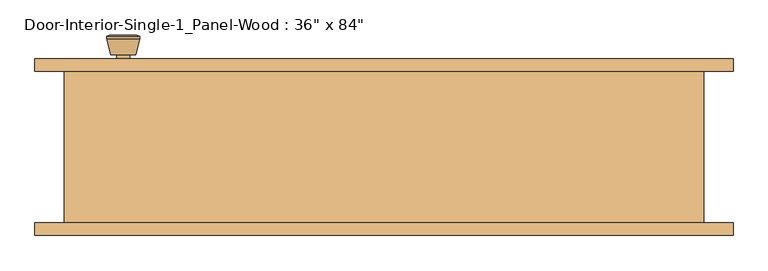
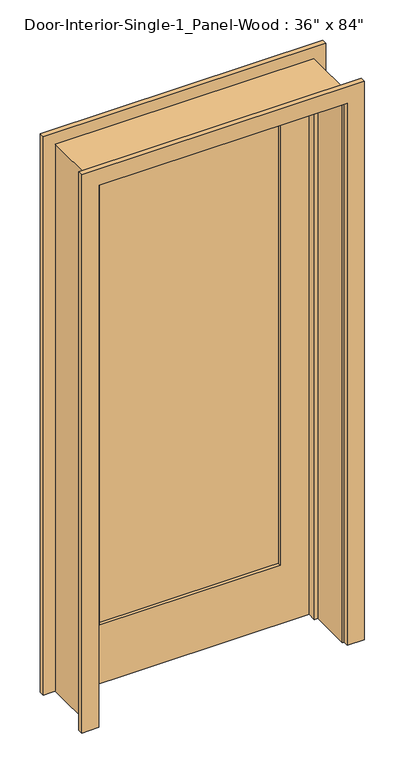
"""IFC4 building model written with IfcOpenShell, lengths in millimetres: door geometry."""

from ifc_helpers import new_model, si_unit, point, frame, frame_2d, origin, place, context, project, spatial, polyline, circle_curve, trimmed, segment, composite_curve, outline, extrude, faceted_brep, source, transform, mapped, element, save
from ifc_brep_helpers import plane_surface, cylinder_surface, revolved_surface, advanced_brep


def door_3b97b8e7(model_context):
    return source(origin(), model_context, "Body", "SolidModel", [
        advanced_brep(
        [(-393.7, 70.2, 914.4), (-383.7, 70.2, 914.4), (-403.7, 70.2, 914.4), (-373.2241324, 21.2, 914.4), (-393.7, 21.2, 914.4), (-414.1758676, 21.2, 914.4), (-368.7, 23.0278681, 914.4), (-418.7, 23.0278681, 914.4), (-368.7, 26.4915463, 914.4), (-418.7, 26.4915463, 914.4), (-375.063764, 51.2, 914.4), (-412.336236, 51.2, 914.4), (-383.7, 51.2, 914.4), (-403.7, 51.2, 914.4)],
        [
            (0, 1),
            (1, 2, circle_curve(frame((-393.7, 70.2, 914.4), z_axis=(0.0, 1.0, 0.0), x_axis=(-1.0, 0.0, 0.0)), 10.0)),
            (2, 0),
            (2, 1, circle_curve(frame((-393.7, 70.2, 914.4), z_axis=(0.0, 1.0, 0.0), x_axis=(-1.0, 0.0, 0.0)), 10.0)),
            (3, 4),
            (4, 5),
            (5, 3, circle_curve(frame((-393.7, 21.2, 914.4), z_axis=(0.0, -1.0, 0.0), x_axis=(-1.0, 0.0, 0.0)), 20.4758676)),
            (3, 5, circle_curve(frame((-393.7, 21.2, 914.4), z_axis=(0.0, -1.0, 0.0), x_axis=(-1.0, 0.0, 0.0)), 20.4758676)),
            (6, 3),
            (5, 7),
            (7, 6, circle_curve(frame((-393.7, 23.0278681, 914.4), z_axis=(0.0, -1.0, 0.0), x_axis=(-1.0, 0.0, 0.0)), 25.0)),
            (6, 7, circle_curve(frame((-393.7, 23.0278681, 914.4), z_axis=(0.0, -1.0, 0.0), x_axis=(-1.0, 0.0, 0.0)), 25.0)),
            (8, 6),
            (7, 9),
            (9, 8, circle_curve(frame((-393.7, 26.4915463, 914.4), z_axis=(0.0, -1.0, 0.0), x_axis=(-1.0, 0.0, 0.0)), 25.0)),
            (8, 9, circle_curve(frame((-393.7, 26.4915463, 914.4), z_axis=(0.0, -1.0, 0.0), x_axis=(-1.0, 0.0, 0.0)), 25.0)),
            (10, 8),
            (9, 11),
            (11, 10, circle_curve(frame((-393.7, 51.2, 914.4), z_axis=(0.0, -1.0, 0.0), x_axis=(-1.0, 0.0, 0.0)), 18.636236)),
            (10, 11, circle_curve(frame((-393.7, 51.2, 914.4), z_axis=(0.0, -1.0, 0.0), x_axis=(-1.0, 0.0, 0.0)), 18.636236)),
            (12, 10),
            (11, 13),
            (13, 12, circle_curve(frame((-393.7, 51.2, 914.4), z_axis=(0.0, -1.0, 0.0), x_axis=(-1.0, 0.0, 0.0)), 10.0)),
            (12, 13, circle_curve(frame((-393.7, 51.2, 914.4), z_axis=(0.0, -1.0, 0.0), x_axis=(-1.0, 0.0, 0.0)), 10.0)),
            (1, 12),
            (13, 2),
        ],
        [
            plane_surface(frame((-393.7, 70.2, 914.4), z_axis=(0.0, 1.0, 0.0), x_axis=(-1.0, 0.0, 0.0))),
            plane_surface(frame((-393.7, 21.2, 914.4), z_axis=(0.0, -1.0, 0.0), x_axis=(-1.0, 0.0, 0.0))),
            revolved_surface(polyline([(-414.1758676, 21.2, 914.4), (-418.7, 23.0278681, 914.4)]), (-393.7, 70.2, 914.4), (0.0, 1.0, 0.0)),
            cylinder_surface(frame((-393.7, 70.2, 914.4), z_axis=(0.0, 1.0, 0.0), x_axis=(-1.0, 0.0, 0.0)), 25.0),
            revolved_surface(polyline([(-418.7, 26.4915463, 914.4), (-412.336236, 51.2, 914.4)]), (-393.7, 70.2, 914.4), (0.0, 1.0, 0.0)),
            plane_surface(frame((-393.7, 51.2, 914.4), z_axis=(0.0, 1.0, 0.0), x_axis=(-1.0, 0.0, 0.0))),
            cylinder_surface(frame((-393.7, 70.2, 914.4), z_axis=(0.0, 1.0, 0.0), x_axis=(-1.0, 0.0, 0.0)), 10.0),
        ],
        [
            (0, [[1, 2, 3]]),
            (0, [[-3, 4, -1]]),
            (1, [[5, 6, 7]]),
            (1, [[-6, -5, 8]]),
            (2, [[9, -7, 10, 11]]),
            (2, [[-10, -8, -9, 12]]),
            (3, [[13, -11, 14, 15]]),
            (3, [[-14, -12, -13, 16]]),
            (4, [[17, -15, 18, 19]]),
            (4, [[-18, -16, -17, 20]]),
            (5, [[21, -19, 22, 23]]),
            (5, [[-22, -20, -21, 24]]),
            (6, [[25, -23, 26, -2]]),
            (6, [[-26, -24, -25, -4]]),
        ],
    ),
        extrude(outline(composite_curve([segment(trimmed(circle_curve(frame_2d((914.4, -393.7)), 30.0), [point((914.4, -423.7))], [point((914.4, -363.7))], False, "CARTESIAN"), True, "CONTINUOUS"), segment(trimmed(circle_curve(frame_2d((914.4, -393.7)), 30.0), [point((914.4, -363.7))], [point((914.4, -423.7))], False, "CARTESIAN"), True, "CONTINUOUS")], self_intersect=False)), frame((0.0, 70.2, 0.0), z_axis=(0.0, 1.0, 0.0), x_axis=(0.0, 0.0, 1.0)), (0.0, 0.0, 1.0), 6.0),
        advanced_brep(
        [(-393.7, 117.125, 914.4), (-403.7, 117.125, 914.4), (-383.7, 117.125, 914.4), (-373.2241324, 166.125, 914.4), (-414.1758676, 166.125, 914.4), (-393.7, 166.125, 914.4), (-368.7, 164.2971319, 914.4), (-418.7, 164.2971319, 914.4), (-368.7, 160.8334537, 914.4), (-418.7, 160.8334537, 914.4), (-375.063764, 136.125, 914.4), (-412.336236, 136.125, 914.4), (-383.7, 136.125, 914.4), (-403.7, 136.125, 914.4)],
        [
            (0, 1),
            (1, 2, circle_curve(frame((-393.7, 117.125, 914.4), z_axis=(0.0, -1.0, 0.0), x_axis=(-1.0, 0.0, 0.0)), 10.0)),
            (2, 0),
            (2, 1, circle_curve(frame((-393.7, 117.125, 914.4), z_axis=(0.0, -1.0, 0.0), x_axis=(-1.0, 0.0, 0.0)), 10.0)),
            (3, 4, circle_curve(frame((-393.7, 166.125, 914.4), z_axis=(0.0, 1.0, 0.0), x_axis=(-1.0, 0.0, 0.0)), 20.4758676)),
            (4, 5),
            (5, 3),
            (4, 3, circle_curve(frame((-393.7, 166.125, 914.4), z_axis=(0.0, 1.0, 0.0), x_axis=(-1.0, 0.0, 0.0)), 20.4758676)),
            (6, 7, circle_curve(frame((-393.7, 164.2971319, 914.4), z_axis=(0.0, 1.0, 0.0), x_axis=(-1.0, 0.0, 0.0)), 25.0)),
            (7, 4),
            (3, 6),
            (7, 6, circle_curve(frame((-393.7, 164.2971319, 914.4), z_axis=(0.0, 1.0, 0.0), x_axis=(-1.0, 0.0, 0.0)), 25.0)),
            (8, 9, circle_curve(frame((-393.7, 160.8334537, 914.4), z_axis=(0.0, 1.0, 0.0), x_axis=(-1.0, 0.0, 0.0)), 25.0)),
            (9, 7),
            (6, 8),
            (9, 8, circle_curve(frame((-393.7, 160.8334537, 914.4), z_axis=(0.0, 1.0, 0.0), x_axis=(-1.0, 0.0, 0.0)), 25.0)),
            (10, 11, circle_curve(frame((-393.7, 136.125, 914.4), z_axis=(0.0, 1.0, 0.0), x_axis=(-1.0, 0.0, 0.0)), 18.636236)),
            (11, 9),
            (8, 10),
            (11, 10, circle_curve(frame((-393.7, 136.125, 914.4), z_axis=(0.0, 1.0, 0.0), x_axis=(-1.0, 0.0, 0.0)), 18.636236)),
            (12, 13, circle_curve(frame((-393.7, 136.125, 914.4), z_axis=(0.0, 1.0, 0.0), x_axis=(-1.0, 0.0, 0.0)), 10.0)),
            (13, 11),
            (10, 12),
            (13, 12, circle_curve(frame((-393.7, 136.125, 914.4), z_axis=(0.0, 1.0, 0.0), x_axis=(-1.0, 0.0, 0.0)), 10.0)),
            (1, 13),
            (12, 2),
        ],
        [
            plane_surface(frame((-393.7, 117.125, 914.4), z_axis=(0.0, -1.0, 0.0), x_axis=(-1.0, 0.0, 0.0))),
            plane_surface(frame((-393.7, 166.125, 914.4), z_axis=(0.0, 1.0, 0.0), x_axis=(-1.0, 0.0, 0.0))),
            revolved_surface(polyline([(-414.1758676, 166.125, 914.4), (-418.7, 164.2971319, 914.4)]), (-393.7, 117.125, 914.4), (0.0, -1.0, 0.0)),
            cylinder_surface(frame((-393.7, 117.125, 914.4), z_axis=(0.0, -1.0, 0.0), x_axis=(-1.0, 0.0, 0.0)), 25.0),
            revolved_surface(polyline([(-418.7, 160.8334537, 914.4), (-412.336236, 136.125, 914.4)]), (-393.7, 117.125, 914.4), (0.0, -1.0, 0.0)),
            plane_surface(frame((-393.7, 136.125, 914.4), z_axis=(0.0, -1.0, 0.0), x_axis=(-1.0, 0.0, 0.0))),
            cylinder_surface(frame((-393.7, 117.125, 914.4), z_axis=(0.0, -1.0, 0.0), x_axis=(-1.0, 0.0, 0.0)), 10.0),
        ],
        [
            (0, [[1, 2, 3]]),
            (0, [[-3, 4, -1]]),
            (1, [[5, 6, 7]]),
            (1, [[8, -7, -6]]),
            (2, [[9, 10, -5, 11]]),
            (2, [[12, -11, -8, -10]]),
            (3, [[13, 14, -9, 15]]),
            (3, [[16, -15, -12, -14]]),
            (4, [[17, 18, -13, 19]]),
            (4, [[20, -19, -16, -18]]),
            (5, [[21, 22, -17, 23]]),
            (5, [[24, -23, -20, -22]]),
            (6, [[-2, 25, -21, 26]]),
            (6, [[-4, -26, -24, -25]]),
        ],
    ),
        extrude(outline(composite_curve([segment(trimmed(circle_curve(frame_2d((914.4, -393.7)), 30.0), [point((914.4, -423.7))], [point((914.4, -363.7))], False, "CARTESIAN"), True, "CONTINUOUS"), segment(trimmed(circle_curve(frame_2d((914.4, -393.7)), 30.0), [point((914.4, -363.7))], [point((914.4, -423.7))], False, "CARTESIAN"), True, "CONTINUOUS")], self_intersect=False)), frame((0.0, 111.125, 0.0), z_axis=(0.0, 1.0, 0.0), x_axis=(0.0, 0.0, 1.0)), (0.0, 0.0, 1.0), 6.0),
        faceted_brep([(482.6, 111.125, 0.0), (482.6, -117.475, 0.0), (457.2, -117.475, 0.0), (457.2, 41.275, 0.0), (444.5, 41.275, 0.0), (444.5, 76.2, 0.0), (457.2, 76.2, 0.0), (457.2, 111.125, 0.0), (482.6, 111.125, 2159.0), (482.6, -117.475, 2159.0), (-482.6, -117.475, 2159.0), (-482.6, -117.475, 0.0), (-457.2, -117.475, 0.0), (-457.2, -117.475, 2133.6), (457.2, -117.475, 2133.6), (457.2, 41.275, 2133.6), (-457.2, 41.275, 2133.6), (-457.2, 41.275, 0.0), (-444.5, 41.275, 0.0), (-444.5, 41.275, 2120.9), (444.5, 41.275, 2120.9), (444.5, 76.2, 2120.9), (-444.5, 76.2, 2120.9), (-444.5, 76.2, 0.0), (-457.2, 76.2, 0.0), (-457.2, 76.2, 2133.6), (457.2, 76.2, 2133.6), (457.2, 111.125, 2133.6), (-457.2, 111.125, 2133.6), (-457.2, 111.125, 0.0), (-482.6, 111.125, 0.0), (-482.6, 111.125, 2159.0)], [[[0, 1, 2, 3, 4, 5, 6, 7]], [[1, 0, 8, 9]], [[2, 1, 9, 10, 11, 12, 13, 14]], [[3, 2, 14, 15]], [[4, 3, 15, 16, 17, 18, 19, 20]], [[5, 4, 20, 21]], [[6, 5, 21, 22, 23, 24, 25, 26]], [[7, 6, 26, 27]], [[0, 7, 27, 28, 29, 30, 31, 8]], [[9, 8, 31, 10]], [[15, 14, 13, 16]], [[21, 20, 19, 22]], [[27, 26, 25, 28]], [[30, 29, 24, 23, 18, 17, 12, 11]], [[10, 31, 30, 11]], [[16, 13, 12, 17]], [[22, 19, 18, 23]], [[28, 25, 24, 29]]]),
        extrude(outline(polyline([(2133.6, -457.2), (0.0, -457.2), (0.0, 457.2), (2133.6, 457.2), (2133.6, -457.2)]), holes=[polyline([(2014.5375, -336.55), (2014.5375, 336.55), (231.775, 336.55), (231.775, -336.55), (2014.5375, -336.55)])]), frame((0.0, 76.2, 0.0), z_axis=(0.0, 1.0, 0.0), x_axis=(0.0, 0.0, 1.0)), (0.0, 0.0, 1.0), 34.925),
        extrude(outline(polyline([(336.55, 87.8416667), (-336.55, 87.8416667), (-336.55, 99.4833333), (336.55, 99.4833333), (336.55, 87.8416667)])), frame((0.0, 0.0, 231.775), z_axis=(0.0, 0.0, 1.0), x_axis=(1.0, 0.0, 0.0)), (0.0, 0.0, 1.0), 1782.7625),
        extrude(outline(polyline([(0.0, 463.55), (0.0, 527.05), (2203.45, 527.05), (2203.45, -527.05), (0.0, -527.05), (0.0, -463.55), (2139.95, -463.55), (2139.95, 463.55), (0.0, 463.55)])), frame((0.0, 111.125, 0.0), z_axis=(0.0, 1.0, 0.0), x_axis=(0.0, 0.0, 1.0)), (0.0, 0.0, 1.0), 19.05),
        extrude(outline(polyline([(0.0, 463.55), (0.0, 527.05), (2203.45, 527.05), (2203.45, -527.05), (0.0, -527.05), (0.0, -463.55), (2139.95, -463.55), (2139.95, 463.55), (0.0, 463.55)])), frame((0.0, -136.525, 0.0), z_axis=(0.0, 1.0, 0.0), x_axis=(0.0, 0.0, 1.0)), (0.0, 0.0, 1.0), 19.05),
    ])


if __name__ == "__main__":
    model = new_model("IFC4")
    model_context = context("Model", 3, world=origin())
    ifc_project = project(units=[si_unit("LENGTHUNIT", "METRE", prefix="MILLI")], contexts=[model_context])
    site = spatial("IfcSite", under=ifc_project)
    building = spatial("IfcBuilding", under=site)
    placement = place(None, origin())
    door_shape = door_3b97b8e7(model_context)
    element("IfcDoor", 1, ObjectType="Door-Interior-Single-1_Panel-Wood : 36\" x 84\"", at=placement, inside=building, context=model_context, shape_type="MappedRepresentation", body=[
        mapped(door_shape, transform((0.0, 0.0, 0.0), x_axis=(1.0, 0.0, 0.0), y_axis=(0.0, 1.0, 0.0), z_axis=(0.0, 0.0, 1.0))),
    ])
    save(model, "model.ifc")

# Revit data of these elements
# Type "Door-Interior-Single-1_Panel-Wood : 36\" x 84\""
#   Type Mark = "8"
#   Assembly Code = "C1020300"
#   Analytic Construction = "Wooden"
#   Top Rail = 0' - 4 11/16"
#   Thickness = 0' - 1 3/8"
#   Thermal Resistance (R) = 2.5876 (h·ft²·°F)/BTU
#   Swing Angle [instance default] = 90.00°
#   Stiles = 0' - 4 3/4"
#   Rough Width = 3' - 2"
#   Rough Height = 7' - 1"
#   Height = 7' - 0"
#   Width = 3' - 0"
#   Heat Transfer Coefficient (U) = 0.3865 BTU/(h·ft²·°F)
#   Bottom Rail = 0' - 9 1/8"
#   Trim Material = Cherry
#   Panel Material = Cherry
#   Frame Material = Cherry
#   Door Handle Material = Aluminum
#   Visual Light Transmittance = 0
#   Solar Heat Gain Coefficient = 0
#   Wall Closure = (empty or 0)
#   Function = (empty or 0)
# Element 1 (IfcDoor, "Door-Interior-Single-1_Panel-Wood : 36\" x 84\"")
#   Materials on its faces: "Cherry", "Aluminum"
# Materials
#   "Cherry": class "Wood", colour RGB 226 177 128, transparency 0, Description = "Prunus Serotina", Cost = 0
#   "Aluminum": class "Metal", colour RGB 247 247 247, transparency 0, Description = "Aluminum 6061", Cost = 0
